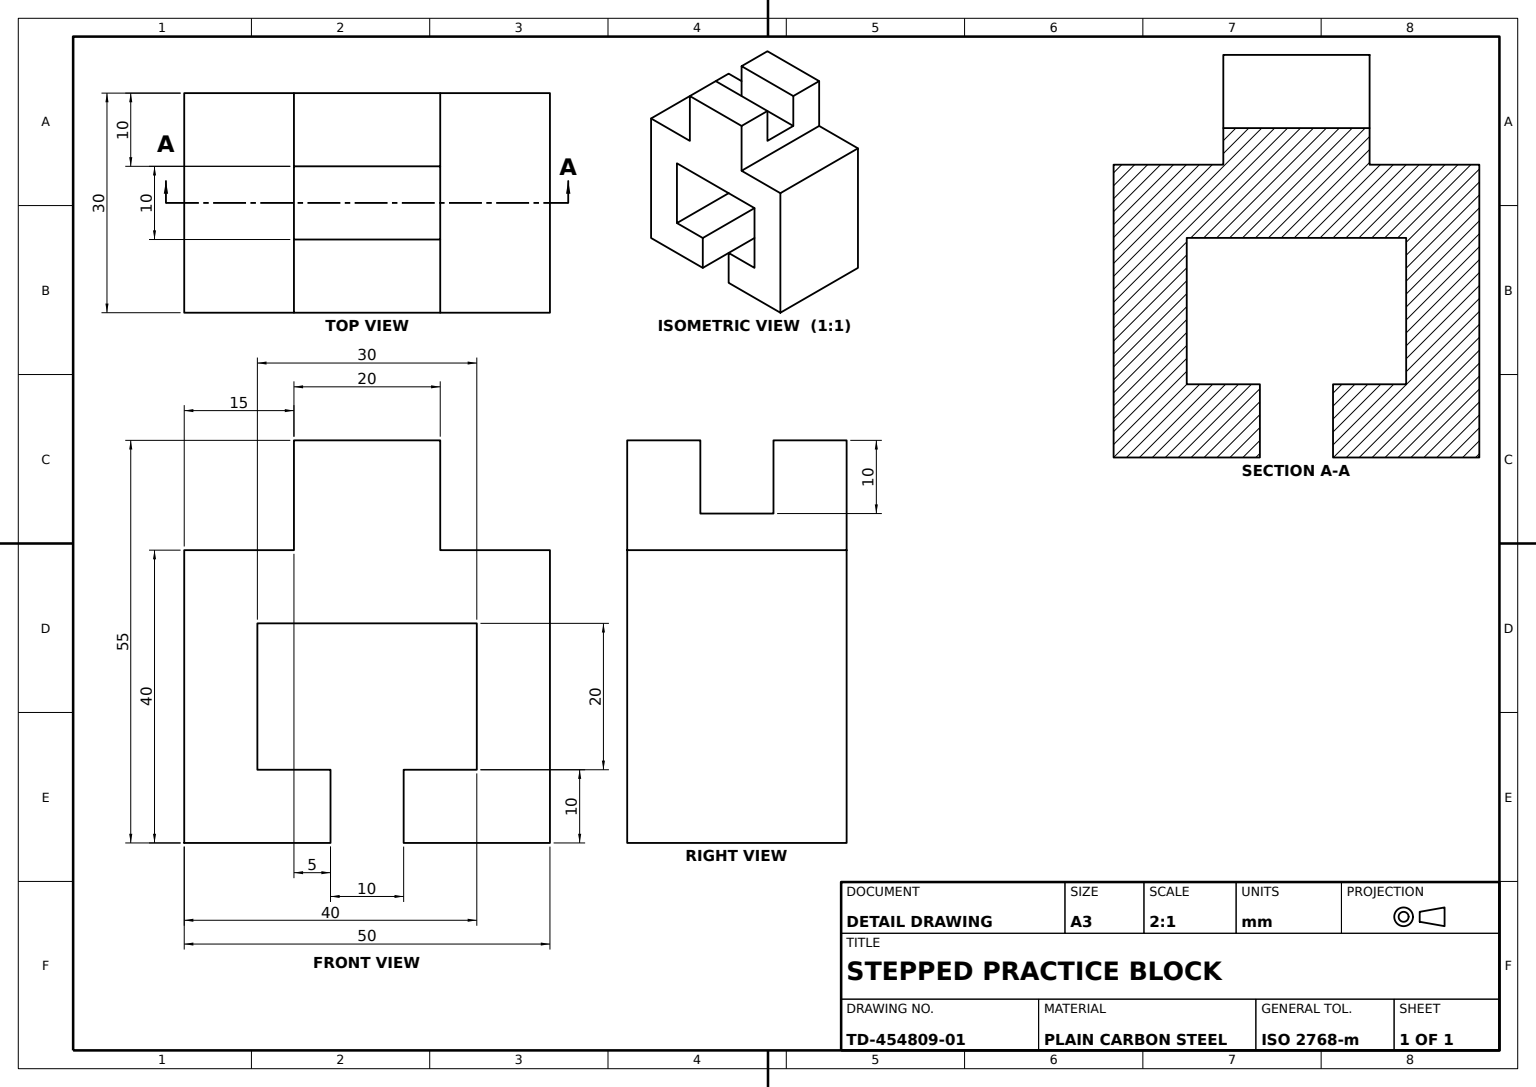
from build123d import *

# Parameters (mm, degrees)
BLOCK_BODY_EXTRUDE_30MM_DEPTH = 30
POCKET_SKETCH_W               = 20
POCKET_SKETCH_H               = 10
POCKET_CUT_10MM_DEPTH         = 10


with BuildPart() as part:
    # Block Profile Sketch → Block Body Extrude 30mm (new body)
    with BuildSketch(Plane.XY):
        Polygon((0, 0), (0, 40), (15, 40), (15, 55), (35, 55), (35, 40), (50, 40), (50, 0), (30, 0), (30, 10), (40, 10), (40, 30), (10, 30), (10, 10), (20, 10), (20, 0), align=None)
    extrude(amount=BLOCK_BODY_EXTRUDE_30MM_DEPTH)

    # Pocket Sketch → Pocket Cut 10mm (cut)
    with BuildSketch(Plane(origin=(0, 55, 0), x_dir=(1, 0, 0), z_dir=(0, 1, 0))):
        with Locations((25, -15)):
            Rectangle(POCKET_SKETCH_W, POCKET_SKETCH_H)
    extrude(amount=-POCKET_CUT_10MM_DEPTH, mode=Mode.SUBTRACT)


solid = part.part
